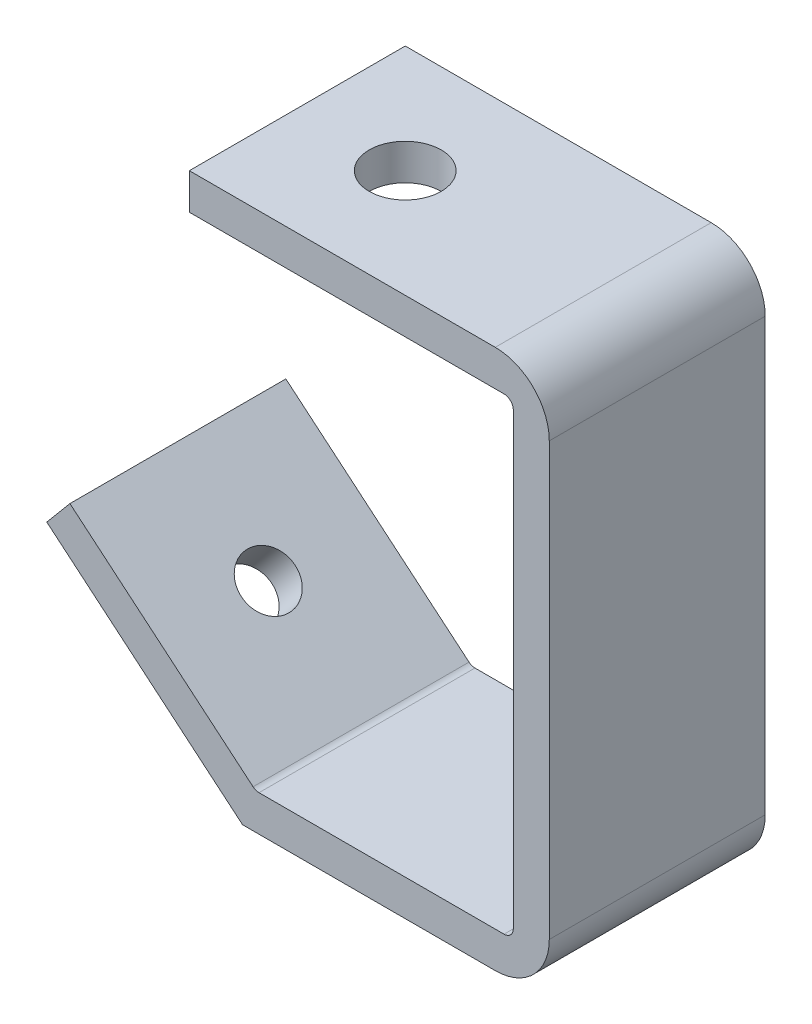
SolidWorks part; units mm, degrees
material "Plain Carbon Steel"
ref_plane "Front Plane" through (0, 0, 0) normal (0, 0, 1) x (1, 0, 0)
ref_plane "Top Plane" through (0, 0, 0) normal (0, 1, 0) x (1, 0, 0)
ref_plane "Right Plane" through (0, 0, 0) normal (1, 0, 0) x (0, 0, -1)
sketch "Bracket Profile Sketch" plane through (0, 0, 0) normal (0, 0, 1) x (1, 0, 0)
  line L0 (0, 0) -> (44.59, 0)
  line L1 (54.12, 9.53) -> (54.12, 85.72)
  line L2 (44.59, 95.25) -> (-9.39, 95.25)
  line L3 (-9.39, 95.25) -> (-9.39, 88.9)
  line L4 (-9.39, 88.9) -> (47.77, 88.9)
  line L5 (47.77, 88.9) -> (47.77, 6.35)
  line L6 (47.77, 6.35) -> (2.3112, 6.35)
  line L7 (2.3112, 6.35) -> (-30.4592, 33.8477)
  line L8 (-30.4592, 33.8477) -> (-34.5409, 28.9833)
  line L9 (-34.5409, 28.9833) -> (0, 0)
  arc A0 (54.12, 9.53) -> (44.59, 0) centre (44.59, 9.53) cw
  arc A1 (54.12, 85.72) -> (44.59, 95.25) centre (44.59, 85.72) ccw
  point P13 (54.12, 0)
  point P16 (54.12, 95.25)
  dimension "D6" = 9.53
  dimension "D1" = 140
  dimension "D2" = 45.09
  dimension "D3" = 63.51
  dimension "D4" = 54.12
  dimension "D5" = 95.25
  dimension "D7" = 6.35
  dimension "D8" = 6.35
  dimension "D9" = 6.35
  dimension "D10" = 6.35
extrude "Bracket Body" add sketch "Bracket Profile Sketch" along normal mid plane 38.1
sketch "Flange Hole A Sketch" plane through (0, 95.25, 0) normal (0, 1, 0) x (1, 0, 0)
  line L0 (-9.39, -19.05) -> (-9.39, 19.05) construction
  circle A0 centre (9.65, 0) radius 6.35
  dimension "D1" = 12.7
  dimension "D2" = 19.04
extrude "Flange Hole A" cut sketch "Flange Hole A Sketch" against normal mid plane 38.1
sketch "Flange Hole B Sketch" plane through (0, 0, 0) normal (-0.6428, -0.766, 0) x (0.766, -0.6428, 0)
  circle A0 centre (-24.28, 0) radius 4.765
  dimension "D1" = 9.53
  dimension "D2" = 20.81
extrude "Flange Hole B" cut sketch "Flange Hole B Sketch" against normal mid plane 38.1
fillet "Bend Fillet R1.63 A" radius 1.63 2 edges at (47.77, 88.9, 0) (47.77, 6.35, 0)
fillet "Bend Fillet R1.63 B" radius 1.63 1 edges at (2.3112, 6.35, 0)
